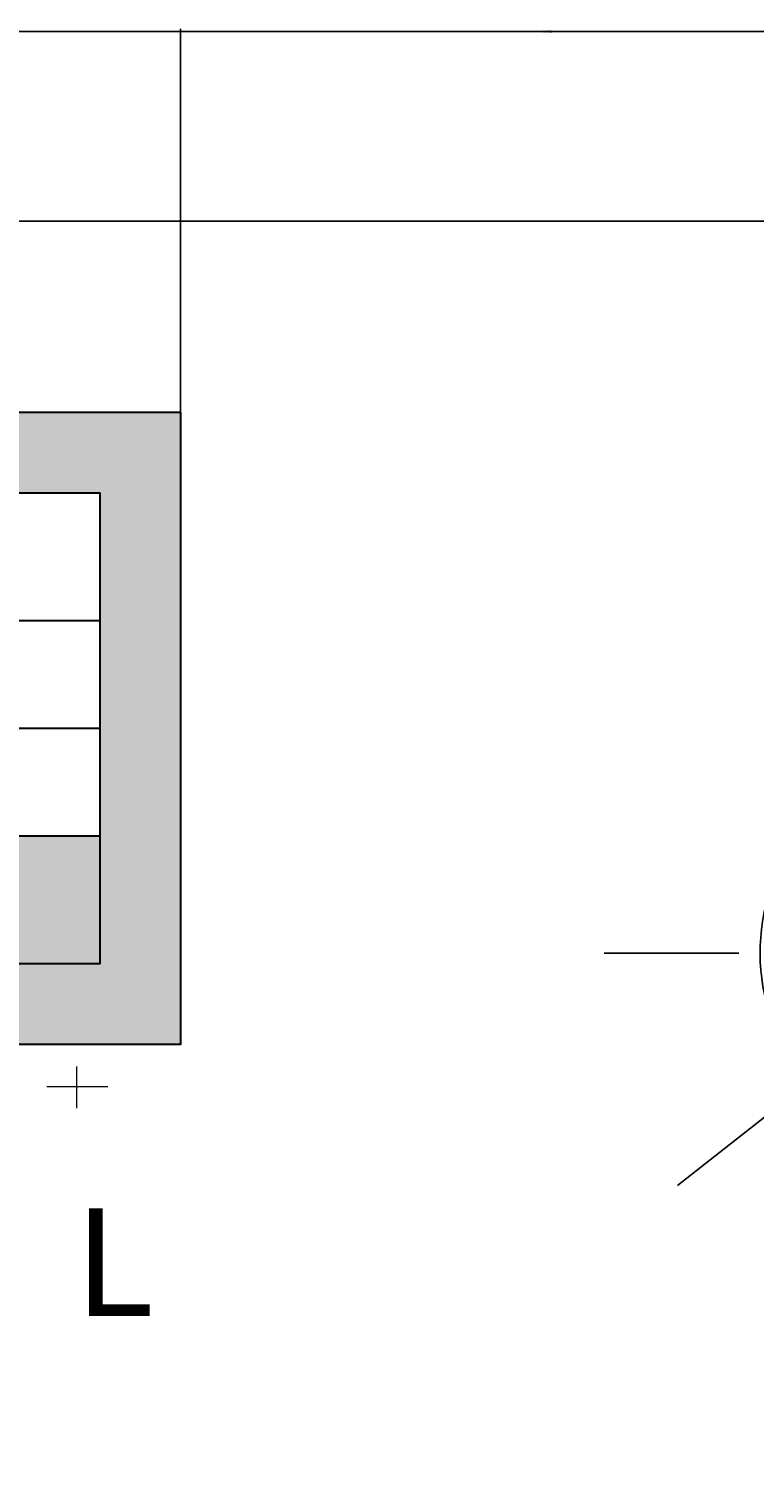
# Model space of a CAD drawing. Units: millimetres. Extents: x -8 to 285, y 5 to 221.
# Tile 15 of 30: x 76 to 130, y 113 to 221. Entities that reach past the tile are written whole.
import ezdxf

# ---------------------------------------------------------------- set-up
doc = ezdxf.new("R2010")
doc.units = ezdxf.units.MM
for name, color, linetype, lineweight in [('A-ANNO-DIMS', 2, 'Continuous', 18), ('E-ANNO-SYMB', 7, 'Continuous', 18), ('E-ANNO-TEXT', 7, 'Continuous', 18), ('E-EQPM-PATT', 252, 'Continuous', 13), ('E-LITE-FIXT', 7, 'Continuous', 25), ('E-POWR-PV', 7, 'Continuous', 30)]:
    doc.layers.add(name, color=color, linetype=linetype, lineweight=lineweight)
doc.styles.get("Standard").update_dxf_attribs({"font": 'arial.ttf'})
doc.dimstyles.get("Standard").update_dxf_attribs({"dimtxt": 0.18, "dimasz": 0.18, "dimexe": 0.18, "dimexo": 0.0625, "dimgap": 0.09, "dimtad": 0, "dimtih": 1, "dimtoh": 1, "dimdec": 4, "dimzin": 0, "dimdsep": 46, "dimtxsty": 'Standard', "dimcen": 0.09, "dimadec": 0, "dimazin": 0, "dimtfac": 1, "dimtdec": 4, "dimtofl": 0, "dimtmove": 0, "dimatfit": 3, "dimfxl": 1, "dimtolj": 1, "dimtzin": 0, "dimarcsym": 0})

# ---------------------------------------------------------------- blocks, each defined once
blk = doc.blocks.new('PV-MODULE-12V')
for p, q in [((18.5, 41), (18.5, 6)), ((6, 31.5), (31, 31.5)), ((6, 23.5), (31, 23.5)), ((6, 15.5), (31, 15.5))]:
    blk.add_line(p, q)
for points in [[(0, 47), (37, 47), (37, 0), (0, 0)], [(6, 41), (31, 41), (31, 6), (6, 6)]]:
    blk.add_lwpolyline(points, close=True)
blk = doc.blocks.new('LAMP-INCANDESCENT')
for p, q in [((7.41, 29.99), (10.59, 43.04)), ((23.41, 29.99), (18.59, 43.04)), ((9.73, 39.52), (19.89, 39.52)), ((9, 36.52), (21, 36.52)), ((8.27, 33.52), (22.11, 33.52)), ((7.41, 29.99), (7.41, 27.94)), ((12.67, 29.99), (8.83, 14.29)), ((22.32, 14.9), (18.15, 29.99)), ((23.41, 29.99), (23.41, 27.42)), ((8.83, 14.29), (13.57, 17.03)), ((13.57, 17.03), (17.07, 15.01)), ((17.07, 15.01), (18.33, 17.21)), ((18.33, 17.21), (22.32, 14.9))]:
    blk.add_line(p, q)
for points in [[(10.59, 43.04), (18.59, 43.04)], [(23.41, 29.99), (7.41, 29.99)]]:
    blk.add_lwpolyline(points)
for centre, radius, start, end in [((14.59, 43.04), 4, 0, 180), ((15, 15), 15, 88.4488, 91.5512), ((15, 15), 15, 120.4152, 55.9163)]:
    blk.add_arc(centre, radius, start, end)
blk = doc.blocks.new('POLARITY-POSITIVE')
for p, q in [((2.22, 3.09), (2.22, 0)), ((0, 1.6), (4.54, 1.6))]:
    blk.add_line(p, q)
blk = doc.blocks.new('*D9')
at = {"layer": 'A-ANNO-DIMS', "color": 0, "lineweight": -2, "transparency": 16777216}
for p, q in [((6.67, 133.79), (6.67, 220.74)), ((6.85, 220.56), (138.33, 220.56)), ((270.74, 220.56), (139.26, 220.56)), ((270.92, 206.52), (270.92, 220.74))]:
    blk.add_line(p, q, dxfattribs=at)
at = {"layer": 'A-ANNO-DIMS', "color": 0, "transparency": 16777216}
for points in [[(6.85, 220.59), (6.85, 220.53), (6.67, 220.56)], [(270.74, 220.59), (270.74, 220.53), (270.92, 220.56)]]:
    blk.add_solid(points, dxfattribs=at)
at = {"layer": 'Defpoints', "color": 0, "transparency": 16777216}
for p in [(270.92, 220.56), (270.92, 206.46), (6.67, 133.73)]:
    blk.add_point(p, dxfattribs=at)
at = {"layer": 'A-ANNO-DIMS', "color": 0, "transparency": 16777216, "insert": (138.8, 220.56), "char_height": 0.18, "attachment_point": 5}
blk.add_mtext('\\A1;264.25', dxfattribs=at)
blk = doc.blocks.new('*D10')
at = {"layer": 'A-ANNO-DIMS', "color": 0, "lineweight": -2, "transparency": 16777216}
for p, q in [((145.1, 206.46), (-7.61, 206.46)), ((-7.43, 206.28), (-7.43, 113.16)), ((-7.43, 19.68), (-7.43, 112.8)), ((30.45, 19.5), (-7.61, 19.5))]:
    blk.add_line(p, q, dxfattribs=at)
at = {"layer": 'A-ANNO-DIMS', "color": 0, "transparency": 16777216}
for points in [[(-7.46, 206.28), (-7.4, 206.28), (-7.43, 206.46)], [(-7.46, 19.68), (-7.4, 19.68), (-7.43, 19.5)]]:
    blk.add_solid(points, dxfattribs=at)
at = {"layer": 'Defpoints', "color": 0, "transparency": 16777216}
for p in [(-7.43, 206.46), (145.17, 206.46), (30.52, 19.5)]:
    blk.add_point(p, dxfattribs=at)
at = {"layer": 'A-ANNO-DIMS', "color": 0, "transparency": 16777216, "insert": (-7.43, 112.98), "char_height": 0.18, "attachment_point": 5}
blk.add_mtext('\\A1;186.95', dxfattribs=at)
blk = doc.blocks.new('*D12')
at = {"layer": 'A-ANNO-DIMS', "color": 0, "lineweight": -2, "transparency": 16777216}
for p, q in [((87.57, 192.33), (87.57, 220.74)), ((87.75, 220.56), (114.49, 220.56)), ((142.01, 220.56), (115.27, 220.56)), ((142.19, 191.55), (142.19, 220.74))]:
    blk.add_line(p, q, dxfattribs=at)
at = {"layer": 'A-ANNO-DIMS', "color": 0, "transparency": 16777216}
for points in [[(87.75, 220.59), (87.75, 220.53), (87.57, 220.56)], [(142.01, 220.59), (142.01, 220.53), (142.19, 220.56)]]:
    blk.add_solid(points, dxfattribs=at)
at = {"layer": 'Defpoints', "color": 0, "transparency": 16777216}
for p in [(142.19, 220.56), (87.57, 192.27), (142.19, 191.49)]:
    blk.add_point(p, dxfattribs=at)
at = {"layer": 'A-ANNO-DIMS', "color": 0, "transparency": 16777216, "insert": (114.88, 220.56), "char_height": 0.18, "attachment_point": 5}
blk.add_mtext('\\A1;54.62', dxfattribs=at)

msp = doc.modelspace()

# ---------------------------------------------------------------- hatches: boundary and pattern name
at = {"layer": 'E-EQPM-PATT'}
h = msp.add_hatch(color=256, dxfattribs=at)
h.set_gradient(color2=(0, 0, 0), tint=1)
h.paths.add_polyline_path([(6.8535, 192.2715), (6.8535, 145.2715), (43.8535, 145.2715), (43.8535, 192.2715)])
h.paths.add_polyline_path([(37.8535, 186.2715), (37.8535, 151.2715), (12.8535, 151.2715), (12.8535, 186.2715)], flags=0)
h.paths.add_polyline_path([(50.5716, 145.2715), (87.5716, 145.2715), (87.5716, 192.2715), (50.5716, 192.2715)])
h.paths.add_polyline_path([(56.5716, 186.2715), (81.5716, 186.2715), (81.5716, 151.2715), (56.5716, 151.2715)], flags=0)
h.paths.add_polyline_path([(37.8535, 176.7715), (37.8535, 186.2715), (25.3535, 186.2715), (25.3535, 176.7715)], flags=0)
h.paths.add_polyline_path([(37.8535, 176.7715), (37.8535, 186.2715), (12.8535, 186.2715), (12.8535, 176.7715)], flags=0)
h.paths.add_polyline_path([(25.3535, 160.7715), (37.8535, 160.7715), (37.8535, 186.2715), (25.3535, 186.2715)], flags=0)
h.paths.add_polyline_path([(12.8535, 151.2715), (37.8535, 151.2715), (37.8535, 186.2715), (12.8535, 186.2715)], flags=16)
h.paths.add_polyline_path([(56.5716, 186.2715), (56.5716, 160.7715), (81.5716, 160.7715), (81.5716, 186.2715)], flags=0)
h.paths.add_polyline_path([(56.5716, 151.2715), (81.5716, 151.2715), (81.5716, 186.2715), (56.5716, 186.2715)], flags=16)
h = msp.add_hatch(color=256, dxfattribs=at)
h.set_gradient(color2=(0, 0, 0), tint=1)
h.paths.add_polyline_path([(25.3535, 186.2715), (12.8535, 186.2715), (12.8535, 176.7715), (25.3535, 176.7715)])
h.paths.add_polyline_path([(69.0716, 176.7715), (56.5716, 176.7715), (56.5716, 168.7715), (69.0716, 168.7715)])
h.paths.add_polyline_path([(69.0716, 168.7715), (56.5716, 168.7715), (56.5716, 160.7715), (69.0716, 160.7715)])
h.paths.add_polyline_path([(25.3535, 160.7715), (12.8535, 160.7715), (12.8535, 151.2715), (25.3535, 151.2715)])
h.paths.add_polyline_path([(81.5716, 160.7715), (69.0716, 160.7715), (69.0716, 151.2715), (81.5716, 151.2715)])

# ---------------------------------------------------------------- linework, layer by layer
at = {"layer": 'E-LITE-FIXT'}
for p, q in [((129.0987, 152.0675), (119.0987, 152.0675)), ((132.3949, 140.9643), (124.5373, 134.7789))]:
    msp.add_line(p, q, dxfattribs=at)

# ---------------------------------------------------------------- block references
at = {"layer": 'E-ANNO-SYMB'}
msp.add_blockref('POLARITY-POSITIVE', (77.6252, 140.5473), dxfattribs=at)
at = {"layer": 'E-LITE-FIXT'}
msp.add_blockref('LAMP-INCANDESCENT', (130.689, 137.068), dxfattribs=at)
at = {"layer": 'E-POWR-PV'}
msp.add_blockref('PV-MODULE-12V', (50.5711, 145.271), dxfattribs=at)

# ---------------------------------------------------------------- texts
at = {"layer": 'E-ANNO-TEXT', "insert": (79.675, 133.0886), "char_height": 8, "attachment_point": 1}
msp.add_mtext_dynamic_manual_height_columns('L', width=11.038304, gutter_width=12.5, heights=[0], dxfattribs=at)

# ---------------------------------------------------------------- dimensions: what is measured, and where the dimension line sits
at = {"layer": 'A-ANNO-DIMS'}
for base, p1, p2, picture, middle in [((270.9192, 220.5568), (6.6725, 133.7273), (270.9192, 206.4568), '*D9', (138.7958, 220.5568)), ((142.1909, 220.5568), (87.5716, 192.2715), (142.1909, 191.4908), '*D12', (114.8812, 220.5568))]:
    dim = msp.add_linear_dim(base=base, p1=p1, p2=p2, dimstyle='Standard', override={"dimdec": 2, "dimlfac": 1, "dimrnd": 0, "dimzin": 0, "dimdsep": 46, "dimlunit": 2}, dxfattribs=at)
    dim.commit()
    dim.dimension.update_dxf_attribs({"geometry": picture, "text_midpoint": middle})
dim = msp.add_linear_dim(base=(-7.4275, 206.4568), p1=(30.516, 19.502), p2=(145.1651, 206.4568), angle=90, dimstyle='Standard', override={"dimdec": 2, "dimlfac": 1, "dimrnd": 0, "dimzin": 0, "dimdsep": 46, "dimlunit": 2}, dxfattribs=at)
dim.commit()
dim.dimension.update_dxf_attribs({"geometry": '*D10', "text_midpoint": (-7.4275, 112.9794)})

doc.saveas('drawing.dxf')
